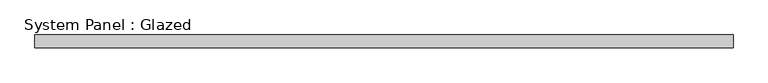
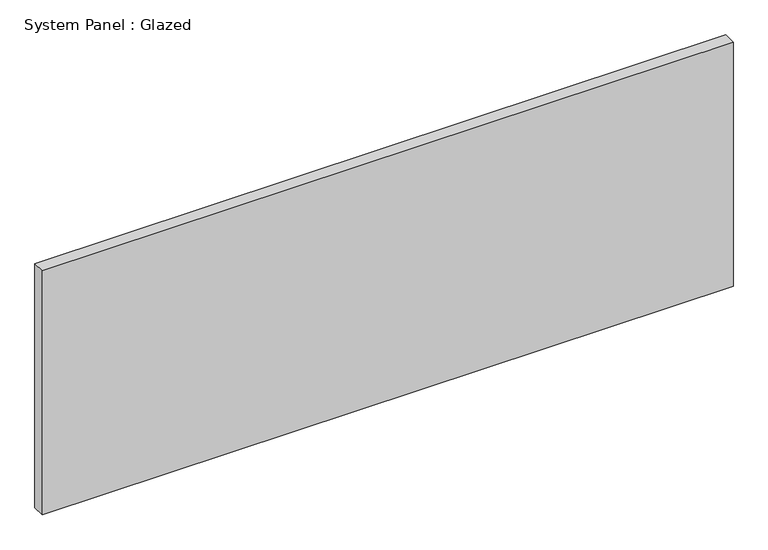
"""IFC4 building model written with IfcOpenShell, lengths in millimetres: plate geometry, System Panel : Glazed."""

from ifc_helpers import new_model, si_unit, origin, origin_with_axes, place, context, project, spatial, polyline, outline, extrude, source, transform, mapped, element, save


def system_panel_glazed_e44632c1(model_context):
    return source(origin(), model_context, "Body", "SweptSolid", [
        extrude(outline(polyline([(688.975, 19.05), (-688.975, 19.05), (-688.975, 44.45), (688.975, 44.45), (688.975, 19.05)])), origin_with_axes(), (0.0, 0.0, 1.0), 514.35),
    ])


if __name__ == "__main__":
    model = new_model("IFC4")
    model_context = context("Model", 3, world=origin())
    ifc_project = project(units=[si_unit("LENGTHUNIT", "METRE", prefix="MILLI")], contexts=[model_context])
    site = spatial("IfcSite", under=ifc_project)
    building = spatial("IfcBuilding", under=site)
    placement = place(None, origin())
    system_panel_glazed_shape = system_panel_glazed_e44632c1(model_context)
    element("IfcPlate", 1, ObjectType="System Panel : Glazed", at=placement, inside=building, context=model_context, shape_type="MappedRepresentation", body=[
        mapped(system_panel_glazed_shape, transform((0.0, 0.0, 0.0), x_axis=(1.0, 0.0, 0.0), y_axis=(0.0, 1.0, 0.0), z_axis=(0.0, 0.0, 1.0))),
    ])
    save(model, "model.ifc")

# Revit data of these elements
# Type "System Panel : Glazed"
#   Construction Type Id = "GSP4R"
#   Analytic Construction = "1/8 in Pilkington single glazing"
#   Visual Light Transmittance = 0.9
#   Solar Heat Gain Coefficient = 0.86
#   Heat Transfer Coefficient (U) = 1.18115 BTU/(h·ft²·°F)
# Element 1 (IfcPlate, "System Panel : Glazed")
#   Materials on its faces: "Glass"
# Materials
#   "Glass": class "Glass", colour RGB 0 128 192, transparency 0.75, Description = "Soda Lime Glass", Cost = 0
